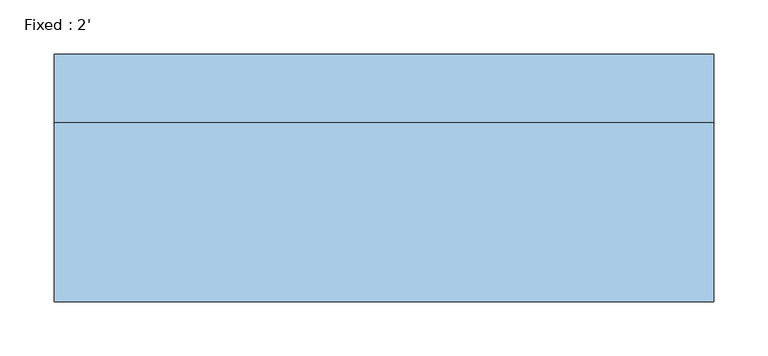
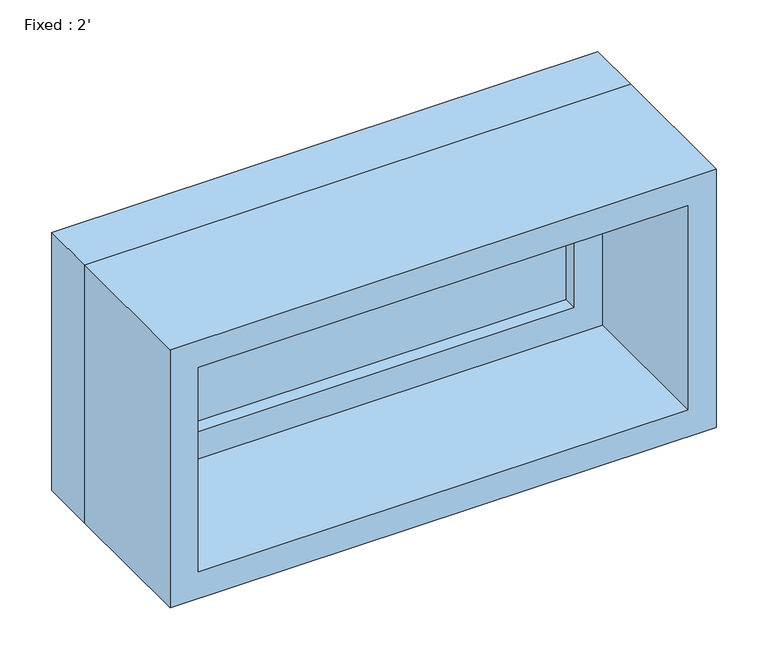
"""IFC4 building model written with IfcOpenShell, lengths in millimetres: window geometry, Fixed : 2'."""

from ifc_helpers import new_model, si_unit, frame, origin, place, context, project, spatial, polyline, outline, extrude, source, transform, mapped, element, save


def fixed_2_d9cafb20(model_context):
    return source(origin(), model_context, "Body", "SweptSolid", [
        extrude(outline(polyline([(203.2, 66.675), (-279.4, 66.675), (-279.4, 79.375), (203.2, 79.375), (203.2, 66.675)])), frame((0.0, 0.0, 2197.1), z_axis=(0.0, 0.0, 1.0), x_axis=(1.0, 0.0, 0.0)), (0.0, 0.0, 1.0), 177.8),
        extrude(outline(polyline([(2419.35, -323.85), (2152.65, -323.85), (2152.65, 247.65), (2419.35, 247.65), (2419.35, -323.85)]), holes=[polyline([(2374.9, -279.4), (2374.9, 203.2), (2197.1, 203.2), (2197.1, -279.4), (2374.9, -279.4)])]), frame((0.0, 50.8, 0.0), z_axis=(0.0, 1.0, 0.0), x_axis=(0.0, 0.0, 1.0)), (0.0, 0.0, 1.0), 44.45),
        extrude(outline(polyline([(2438.4, -342.9), (2133.6, -342.9), (2133.6, 266.7), (2438.4, 266.7), (2438.4, -342.9)]), holes=[polyline([(2406.65, -311.15), (2406.65, 234.95), (2165.35, 234.95), (2165.35, -311.15), (2406.65, -311.15)])]), frame((0.0, -114.3, 0.0), z_axis=(0.0, 1.0, 0.0), x_axis=(0.0, 0.0, 1.0)), (0.0, 0.0, 1.0), 165.1),
        extrude(outline(polyline([(2438.4, 266.7), (2438.4, -342.9), (2133.6, -342.9), (2133.6, 266.7), (2438.4, 266.7)]), holes=[polyline([(2419.35, 247.65), (2152.65, 247.65), (2152.65, -323.85), (2419.35, -323.85), (2419.35, 247.65)])]), frame((0.0, 50.8, 0.0), z_axis=(0.0, 1.0, 0.0), x_axis=(0.0, 0.0, 1.0)), (0.0, 0.0, 1.0), 63.5),
    ])


if __name__ == "__main__":
    model = new_model("IFC4")
    model_context = context("Model", 3, world=origin())
    ifc_project = project(units=[si_unit("LENGTHUNIT", "METRE", prefix="MILLI")], contexts=[model_context])
    site = spatial("IfcSite", under=ifc_project)
    building = spatial("IfcBuilding", under=site)
    placement = place(None, origin())
    fixed_2_shape = fixed_2_d9cafb20(model_context)
    element("IfcWindow", 1, ObjectType="Fixed : 2'", at=placement, inside=building, context=model_context, shape_type="MappedRepresentation", body=[
        mapped(fixed_2_shape, transform((0.0, 0.0, 0.0), x_axis=(1.0, 0.0, 0.0), y_axis=(0.0, 1.0, 0.0), z_axis=(0.0, 0.0, 1.0))),
    ])
    save(model, "model.ifc")

# Revit data of these elements
# Type "Fixed : 2'"
#   Type Mark = "22"
#   Construction Type Id = "GSP4R"
#   Assembly Code = "B2020100"
#   Analytic Construction = "1/8 in Pilkington single glazing"
#   Visual Light Transmittance = 0.9
#   Solar Heat Gain Coefficient = 0.78
#   Heat Transfer Coefficient (U) = 0.6496 BTU/(h·ft²·°F)
#   Height = 1' - 0"
#   Default Sill Height = 7' - 0"
#   Width = 2' - 0"
#   Window Inset = 0' - 0 3/4"
#   Define Thermal Properties by = 1
#   Glass Pane Material = Glass
#   Sash Material = Sash
#   Wall Closure = (empty or 0)
# Element 1 (IfcWindow, "Fixed : 2'")
#   Materials on its faces: "Sash", "Glass"
# Materials
#   "Glass": class "Glass", colour RGB 0 128 192, transparency 0.75, Description = "Soda Lime Glass", Cost = 0
#   "Sash": class "Wood", colour RGB 224 178 126, transparency 0, Cost = 0
